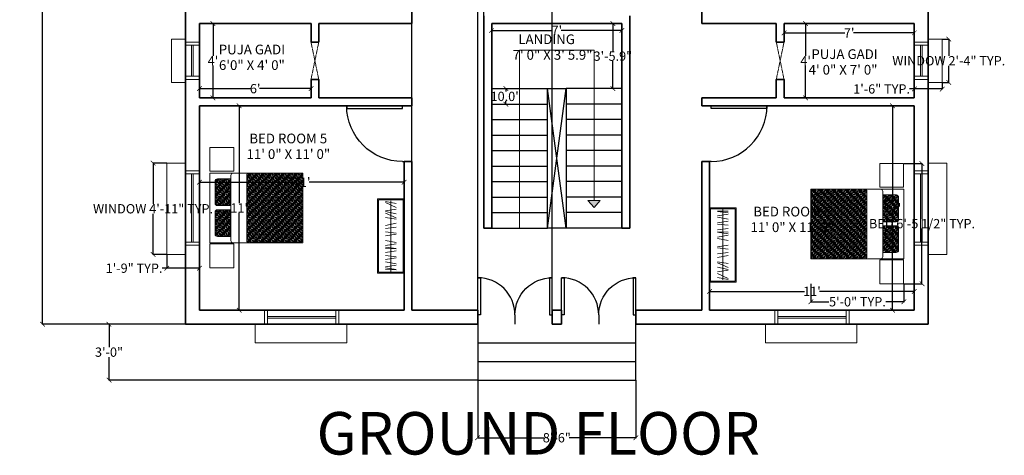
# Model space of a CAD drawing. Units: inches. Extents: x 844 to 2234, y 346 to 1084.
# Tile 1 of 93: x 844 to 1479, y 346 to 627. Entities that reach past the tile are written whole.
import ezdxf

# ---------------------------------------------------------------- set-up
doc = ezdxf.new("R2010")
doc.units = ezdxf.units.IN
doc.header["$MEASUREMENT"] = 0
doc.linetypes.add('DASHED', pattern=[0.75, 0.5, -0.25])
for name, color, linetype, lineweight in [('A-ANNO-DIMS', 2, 'Continuous', 18), ('A-ANNO-SYMB', 7, 'Continuous', 18), ('A-ANNO-TEXT', 7, 'Continuous', 35), ('A-AREA-IDEN', 7, 'Continuous', 18), ('A-FLOR-STRS', 7, 'Continuous', 25), ('A-WALL', 7, 'Continuous', 35), ('A-WALL-OVHD', 7, 'DASHED', 18), ('beds', 130, 'Continuous', 18), ('doors', 170, 'Continuous', 25), ('furniture', 8, 'Continuous', 18), ('windows', 1, 'Continuous', 18)]:
    doc.layers.add(name, color=color, linetype=linetype, lineweight=lineweight)
doc.styles.get("Standard").update_dxf_attribs({"font": 'arial.ttf'})
doc.dimstyles.get("Standard").update_dxf_attribs({"dimtxt": 6, "dimasz": 3, "dimexe": 0.18, "dimexo": 0.0625, "dimgap": 0.09, "dimtad": 0, "dimtih": 1, "dimtoh": 1, "dimdec": 1, "dimzin": 0, "dimdsep": 46, "dimlunit": 3, "dimtxsty": 'Standard', "dimblk": 'ARCHTICK', "dimcen": 0.09, "dimadec": 0, "dimazin": 0, "dimtfac": 1, "dimtdec": 1, "dimtofl": 0, "dimtmove": 0, "dimatfit": 3, "dimfxl": 1, "dimtolj": 1, "dimtzin": 0, "dimarcsym": 0})
pattern_1 = [(135, (-1377.70473, -125.71507), (-0.070710678, -0.070710678), []), (135, (-1377.68705, -125.69739), (-0.070710678, -0.070710678), []), (45, (-1377.70473, -125.71507), (-0.070710678, 0.070710678), [-0.025, 0.025]), (45, (-1377.72241, -125.69739), (-0.070710678, 0.070710678), [-0.025, 0.025]), (45, (-1377.74009, -125.67972), (-0.070710678, 0.070710678), [0.025, -0.025]), (45, (-1377.75776, -125.66204), (-0.070710678, 0.070710678), [0.025, -0.025]), (135, (-1377.66938, -125.67972), (-0.070710678, -0.070710678), [0.025, -0.025]), (135, (-1377.6517, -125.66204), (-0.070710678, -0.070710678), [0.025, -0.025])]

# ---------------------------------------------------------------- blocks, each defined once
blk = doc.blocks.new('*U2')
for p, q in [((0, 0), (0, -6)), ((36, 0), (36, -6))]:
    blk.add_line(p, q)
blk.add_lwpolyline([(0, 0), (0, 36), (1.75, 36), (1.75, 0)], close=True)
blk.add_arc((0, 0), 36, 0, 90)
blk = doc.blocks.new('*U4')
for p, q in [((0, 0), (0, -6)), ((24, 0), (24, -6))]:
    blk.add_line(p, q)
blk.add_lwpolyline([(0, 0), (0, 24), (1.75, 24), (1.75, 0)], close=True)
blk.add_arc((0, 0), 24, 0, 90)
blk = doc.blocks.new('MAT-P10')
h = blk.add_hatch()
h.set_pattern_fill('BOX', color=256, scale=0.1, angle=45, style=0)
h.set_pattern_definition(pattern_1)
h.paths.add_polyline_path([(-0.157, 1.46), (0.417, 1.46), (0.417, 1.751, 0.414214), (0.367, 1.801), (-0.107, 1.801, 0.414214), (-0.157, 1.751)])
h.paths.add_polyline_path([(0.505, 1.46), (1.079, 1.46), (1.079, 1.751, 0.414214), (1.029, 1.801), (0.555, 1.801, 0.414214), (0.505, 1.751)])
h = blk.add_hatch()
h.set_pattern_fill('BOX', color=256, scale=0.1, angle=45, style=0)
h.set_pattern_definition(pattern_1)
edge = h.paths.add_edge_path()
edge.add_line((1.205, -0.085), (1.205, 1.062))
edge.add_ellipse((1.161, 1.063), major_axis=(0, 0.0568), ratio=0.776379, start_angle=270, end_angle=360)
edge.add_line((1.161, 1.119), (-0.251, 1.12))
edge.add_ellipse((-0.251, 1.063), major_axis=(0, 0.0568), ratio=0.776379, start_angle=0, end_angle=88.1396)
edge.add_line((-0.295, 1.064), (-0.295, -0.085))
edge.add_line((-0.295, -0.085), (1.205, -0.085))
for p, q in [((-0.251, 1.46), (1.161, 1.46)), ((-0.251, 1.12), (1.161, 1.119)), ((1.102, 0.406), (1.102, 0.057)), ((1.058, 0), (0.775, 0))]:
    blk.add_line(p, q)
for points in [[(-0.83, 1.909), (-0.319, 1.909), (-0.319, 1.398), (-0.83, 1.398)], [(1.205, -0.085), (-0.295, -0.085), (-0.295, 1.915), (1.205, 1.915)], [(1.244, 1.909), (1.755, 1.909), (1.755, 1.398), (1.244, 1.398)]]:
    blk.add_lwpolyline(points, close=True)
for points in [[(0.417, 1.46), (0.417, 1.751, 0.414214), (0.367, 1.801), (-0.107, 1.801, 0.414214), (-0.157, 1.751), (-0.157, 1.46)], [(1.079, 1.46), (1.079, 1.751, 0.414214), (1.029, 1.801), (0.555, 1.801, 0.414214), (0.505, 1.751), (0.505, 1.46)], [(0.37, 1.624), (0.37, 1.571, -0.414214), (0.32, 1.521), (0.111, 1.521)], [(1.012, 1.644), (1.012, 1.571, -0.414214), (0.962, 1.521), (0.753, 1.521)]]:
    blk.add_lwpolyline(points, format="xyb")
at = {"extrusion": (0, 0, -1)}
for centre, start_param, end_param in [((-0.251, 1.404), 4.712389, 6.283185), ((1.161, 1.404), 0, 1.570796), ((-0.251, 1.063), 4.712389, 6.283185), ((1.161, 1.063), 0, 1.570796), ((1.058, 0.057), 1.570796, 3.141593), ((1.058, 0.057), 1.570796, 3.141593)]:
    blk.add_ellipse(centre, major_axis=(0, 0.0568), ratio=0.776379, start_param=start_param, end_param=end_param, dxfattribs=at)
blk = doc.blocks.new('A$C7A17768A')
for p, q in [((-2.8, 0), (0, 0)), ((-2.8, -1), (-2.8, 0)), ((0, -1), (0, 0)), ((-2.76, -0.04), (-0.04, -0.04)), ((-2.76, -0.96), (-2.76, -0.04)), ((-2.617, -0.3), (-2.694, -0.7)), ((-2.66, -0.7), (-2.466, -0.3)), ((-2.403, -0.3), (-2.342, -0.7)), ((-2.229, -0.296), (-2.317, -0.696)), ((-2.074, -0.3), (-2.25, -0.7)), ((-2.096, -0.7), (-2.033, -0.3)), ((-1.875, -0.3), (-1.796, -0.7)), ((-1.732, -0.3), (-1.675, -0.7)), ((-1.555, -0.7), (-1.507, -0.3)), ((-1.467, -0.3), (-1.403, -0.7)), ((-1.227, -0.7), (-1.151, -0.3)), ((-1.098, -0.3), (-1.034, -0.7)), ((-0.98, -0.7), (-0.921, -0.3)), ((-0.908, -0.3), (-0.919, -0.7)), ((-0.834, -0.3), (-0.777, -0.7)), ((-0.657, -0.7), (-0.61, -0.3)), ((-0.57, -0.3), (-0.505, -0.7)), ((-0.429, -0.7), (-0.353, -0.3)), ((-0.301, -0.3), (-0.237, -0.7)), ((-0.192, -0.7), (-0.133, -0.3)), ((-0.12, -0.3), (-0.131, -0.7)), ((-0.04, -0.96), (-0.04, -0.04)), ((-0.04, -0.5), (-2.716, -0.5)), ((-2.8, -1), (0, -1)), ((-2.76, -0.96), (-0.04, -0.96))]:
    blk.add_line(p, q)
blk = doc.blocks.new('_ArchTick')
at = {"color": 0, "linetype": 'ByBlock', "const_width": 0.15}
blk.add_lwpolyline([(-0.5, -0.5), (0.5, 0.5)], dxfattribs=at)
blk = doc.blocks.new('*D33')
at = {"layer": 'A-ANNO-DIMS', "color": 0, "lineweight": -2, "transparency": 16777216}
for p, q in [((1378.55, 624.31), (1350.37, 624.31)), ((1350.55, 624.31), (1350.55, 603.4)), ((1350.55, 576.31), (1350.55, 597.22)), ((1378.55, 576.31), (1350.37, 576.31))]:
    blk.add_line(p, q, dxfattribs=at)
at = {"layer": 'Defpoints', "color": 0, "transparency": 16777216}
for p in [(1378.62, 624.31), (1350.55, 576.31), (1378.62, 576.31)]:
    blk.add_point(p, dxfattribs=at)
at = {"layer": 'A-ANNO-DIMS', "color": 0, "lineweight": -2, "transparency": 16777216, "xscale": 3, "yscale": 3, "zscale": 3}
for p, rotation in [((1350.55, 624.31), 90), ((1350.55, 576.31), 270)]:
    blk.add_blockref('_ArchTick', p, dxfattribs=dict(at, rotation=rotation))
at = {"layer": 'A-ANNO-DIMS', "color": 0, "transparency": 16777216, "insert": (1350.55, 600.31), "char_height": 6, "attachment_point": 5}
blk.add_mtext("\\A1;4'", dxfattribs=at)
blk = doc.blocks.new('*D34')
at = {"layer": 'A-ANNO-DIMS', "color": 0, "lineweight": -2, "transparency": 16777216}
for p, q in [((1336.62, 618.37), (1336.62, 618.49)), ((1336.62, 618.31), (1375.79, 618.31)), ((1420.62, 618.31), (1381.44, 618.31)), ((1420.62, 618.37), (1420.62, 618.49))]:
    blk.add_line(p, q, dxfattribs=at)
at = {"layer": 'Defpoints', "color": 0, "transparency": 16777216}
for p in [(1336.62, 618.31), (1420.62, 618.31), (1420.62, 618.31)]:
    blk.add_point(p, dxfattribs=at)
at = {"layer": 'A-ANNO-DIMS', "color": 0, "lineweight": -2, "transparency": 16777216, "xscale": 3, "yscale": 3, "zscale": 3, "rotation": 180}
blk.add_blockref('_ArchTick', (1336.62, 618.31), dxfattribs=at)
at = {"layer": 'A-ANNO-DIMS', "color": 0, "lineweight": -2, "transparency": 16777216, "xscale": 3, "yscale": 3, "zscale": 3}
blk.add_blockref('_ArchTick', (1420.62, 618.31), dxfattribs=at)
at = {"layer": 'A-ANNO-DIMS', "color": 0, "transparency": 16777216, "insert": (1378.62, 618.31), "char_height": 6, "attachment_point": 5}
blk.add_mtext("\\A1;7'", dxfattribs=at)
blk = doc.blocks.new('*D35')
at = {"layer": 'A-ANNO-DIMS', "color": 0, "lineweight": -2, "transparency": 16777216}
for p, q in [((959.62, 580.55), (959.62, 582.49)), ((959.62, 582.31), (992.75, 582.31)), ((1031.62, 582.31), (998.48, 582.31)), ((1031.62, 580.55), (1031.62, 582.49))]:
    blk.add_line(p, q, dxfattribs=at)
at = {"layer": 'Defpoints', "color": 0, "transparency": 16777216}
for p in [(959.62, 580.49), (1031.62, 582.31), (1031.62, 580.49)]:
    blk.add_point(p, dxfattribs=at)
at = {"layer": 'A-ANNO-DIMS', "color": 0, "lineweight": -2, "transparency": 16777216, "xscale": 3, "yscale": 3, "zscale": 3, "rotation": 180}
blk.add_blockref('_ArchTick', (959.62, 582.31), dxfattribs=at)
at = {"layer": 'A-ANNO-DIMS', "color": 0, "lineweight": -2, "transparency": 16777216, "xscale": 3, "yscale": 3, "zscale": 3}
blk.add_blockref('_ArchTick', (1031.62, 582.31), dxfattribs=at)
at = {"layer": 'A-ANNO-DIMS', "color": 0, "transparency": 16777216, "insert": (995.62, 582.31), "char_height": 6, "attachment_point": 5}
blk.add_mtext("\\A1;6'", dxfattribs=at)
blk = doc.blocks.new('*D36')
at = {"layer": 'A-ANNO-DIMS', "color": 0, "lineweight": -2, "transparency": 16777216}
for p, q in [((968.62, 624.31), (968.25, 624.31)), ((968.43, 624.31), (968.43, 603.4)), ((968.43, 576.31), (968.43, 597.22)), ((968.62, 576.31), (968.25, 576.31))]:
    blk.add_line(p, q, dxfattribs=at)
at = {"layer": 'Defpoints', "color": 0, "transparency": 16777216}
for p in [(968.68, 624.31), (968.43, 576.31), (968.68, 576.31)]:
    blk.add_point(p, dxfattribs=at)
at = {"layer": 'A-ANNO-DIMS', "color": 0, "lineweight": -2, "transparency": 16777216, "xscale": 3, "yscale": 3, "zscale": 3}
for p, rotation in [((968.43, 624.31), 90), ((968.43, 576.31), 270)]:
    blk.add_blockref('_ArchTick', p, dxfattribs=dict(at, rotation=rotation))
at = {"layer": 'A-ANNO-DIMS', "color": 0, "transparency": 16777216, "insert": (968.43, 600.31), "char_height": 6, "attachment_point": 5}
blk.add_mtext("\\A1;4'", dxfattribs=at)
blk = doc.blocks.new('*D45')
at = {"layer": 'A-ANNO-DIMS', "color": 0, "lineweight": -2, "transparency": 16777216}
for p, q in [((965.15, 571.31), (985.47, 571.31)), ((985.29, 571.31), (985.29, 508.41)), ((985.29, 439.31), (985.29, 502.21)), ((965.15, 439.31), (985.47, 439.31))]:
    blk.add_line(p, q, dxfattribs=at)
at = {"layer": 'Defpoints', "color": 0, "transparency": 16777216}
for p in [(965.09, 571.31), (965.09, 439.31), (985.29, 439.31)]:
    blk.add_point(p, dxfattribs=at)
at = {"layer": 'A-ANNO-DIMS', "color": 0, "lineweight": -2, "transparency": 16777216, "xscale": 3, "yscale": 3, "zscale": 3}
for p, rotation in [((985.29, 571.31), 90), ((985.29, 439.31), 270)]:
    blk.add_blockref('_ArchTick', p, dxfattribs=dict(at, rotation=rotation))
at = {"layer": 'A-ANNO-DIMS', "color": 0, "transparency": 16777216, "insert": (985.29, 505.31), "char_height": 6, "attachment_point": 5}
blk.add_mtext("\\A1;11'", dxfattribs=at)
blk = doc.blocks.new('*D46')
at = {"layer": 'A-ANNO-DIMS', "color": 0, "lineweight": -2, "transparency": 16777216}
for p, q in [((959.62, 520.99), (959.62, 522.08)), ((959.62, 521.9), (1020.72, 521.9)), ((1091.62, 521.9), (1030.51, 521.9)), ((1091.62, 520.99), (1091.62, 522.08))]:
    blk.add_line(p, q, dxfattribs=at)
at = {"layer": 'Defpoints', "color": 0, "transparency": 16777216}
for p in [(959.62, 521.9), (959.62, 520.92), (1091.62, 520.92)]:
    blk.add_point(p, dxfattribs=at)
at = {"layer": 'A-ANNO-DIMS', "color": 0, "lineweight": -2, "transparency": 16777216, "xscale": 3, "yscale": 3, "zscale": 3, "rotation": 180}
blk.add_blockref('_ArchTick', (959.62, 521.9), dxfattribs=at)
at = {"layer": 'A-ANNO-DIMS', "color": 0, "lineweight": -2, "transparency": 16777216, "xscale": 3, "yscale": 3, "zscale": 3}
blk.add_blockref('_ArchTick', (1091.62, 521.9), dxfattribs=at)
at = {"layer": 'A-ANNO-DIMS', "color": 0, "transparency": 16777216, "insert": (1025.62, 521.9), "char_height": 6, "attachment_point": 5}
blk.add_mtext("\\A1;11'", dxfattribs=at)
blk = doc.blocks.new('*D47')
at = {"layer": 'A-ANNO-DIMS', "color": 0, "lineweight": -2, "transparency": 16777216}
for p, q in [((1288.62, 448.97), (1288.62, 451.69)), ((1288.62, 451.51), (1349.72, 451.51)), ((1420.62, 451.51), (1359.51, 451.51)), ((1420.62, 448.97), (1420.62, 451.69))]:
    blk.add_line(p, q, dxfattribs=at)
at = {"layer": 'Defpoints', "color": 0, "transparency": 16777216}
for p in [(1420.62, 451.51), (1288.62, 448.91), (1420.62, 448.91)]:
    blk.add_point(p, dxfattribs=at)
at = {"layer": 'A-ANNO-DIMS', "color": 0, "lineweight": -2, "transparency": 16777216, "xscale": 3, "yscale": 3, "zscale": 3, "rotation": 180}
blk.add_blockref('_ArchTick', (1288.62, 451.51), dxfattribs=at)
at = {"layer": 'A-ANNO-DIMS', "color": 0, "lineweight": -2, "transparency": 16777216, "xscale": 3, "yscale": 3, "zscale": 3}
blk.add_blockref('_ArchTick', (1420.62, 451.51), dxfattribs=at)
at = {"layer": 'A-ANNO-DIMS', "color": 0, "transparency": 16777216, "insert": (1354.62, 451.51), "char_height": 6, "attachment_point": 5}
blk.add_mtext("\\A1;11'", dxfattribs=at)
blk = doc.blocks.new('*D48')
at = {"layer": 'A-ANNO-DIMS', "color": 0, "lineweight": -2, "transparency": 16777216}
for p, q in [((1410.5, 571.31), (1406.35, 571.31)), ((1406.53, 571.31), (1406.53, 508.41)), ((1406.53, 439.31), (1406.53, 502.21)), ((1410.5, 439.31), (1406.35, 439.31))]:
    blk.add_line(p, q, dxfattribs=at)
at = {"layer": 'Defpoints', "color": 0, "transparency": 16777216}
for p in [(1410.56, 571.31), (1406.53, 439.31), (1410.56, 439.31)]:
    blk.add_point(p, dxfattribs=at)
at = {"layer": 'A-ANNO-DIMS', "color": 0, "lineweight": -2, "transparency": 16777216, "xscale": 3, "yscale": 3, "zscale": 3}
for p, rotation in [((1406.53, 571.31), 90), ((1406.53, 439.31), 270)]:
    blk.add_blockref('_ArchTick', p, dxfattribs=dict(at, rotation=rotation))
at = {"layer": 'A-ANNO-DIMS', "color": 0, "transparency": 16777216, "insert": (1406.53, 505.31), "char_height": 6, "attachment_point": 5}
blk.add_mtext("\\A1;11'", dxfattribs=at)
blk = doc.blocks.new('*D50')
at = {"layer": 'A-ANNO-DIMS', "color": 0, "lineweight": -2, "transparency": 16777216}
for p, q in [((1156.79, 582.31), (1157.46, 582.31)), ((1157.28, 582.31), (1157.28, 580.46)), ((1156.79, 572.31), (1157.46, 572.31)), ((1157.28, 572.31), (1157.28, 574.16))]:
    blk.add_line(p, q, dxfattribs=at)
at = {"layer": 'Defpoints', "color": 0, "transparency": 16777216}
for p in [(1156.72, 582.31), (1156.72, 572.31), (1157.28, 572.31)]:
    blk.add_point(p, dxfattribs=at)
at = {"layer": 'A-ANNO-DIMS', "color": 0, "lineweight": -2, "transparency": 16777216, "xscale": 3, "yscale": 3, "zscale": 3}
for p, rotation in [((1157.28, 582.31), 90), ((1157.28, 572.31), 270)]:
    blk.add_blockref('_ArchTick', p, dxfattribs=dict(at, rotation=rotation))
at = {"layer": 'A-ANNO-DIMS', "color": 0, "transparency": 16777216, "insert": (1157.28, 577.31), "char_height": 6, "attachment_point": 5}
blk.add_mtext('\\A1;10.0"', dxfattribs=at)
blk = doc.blocks.new('*D51')
at = {"layer": 'A-ANNO-DIMS', "color": 0, "lineweight": -2, "transparency": 16777216}
for p, q in [((1148.12, 619.91), (1148.12, 620.03)), ((1148.12, 619.85), (1187.29, 619.85)), ((1232.12, 619.85), (1192.94, 619.85)), ((1232.12, 619.91), (1232.12, 620.03))]:
    blk.add_line(p, q, dxfattribs=at)
at = {"layer": 'Defpoints', "color": 0, "transparency": 16777216}
for p in [(1148.12, 619.85), (1232.12, 619.85), (1232.12, 619.85)]:
    blk.add_point(p, dxfattribs=at)
at = {"layer": 'A-ANNO-DIMS', "color": 0, "lineweight": -2, "transparency": 16777216, "xscale": 3, "yscale": 3, "zscale": 3, "rotation": 180}
blk.add_blockref('_ArchTick', (1148.12, 619.85), dxfattribs=at)
at = {"layer": 'A-ANNO-DIMS', "color": 0, "lineweight": -2, "transparency": 16777216, "xscale": 3, "yscale": 3, "zscale": 3}
blk.add_blockref('_ArchTick', (1232.12, 619.85), dxfattribs=at)
at = {"layer": 'A-ANNO-DIMS', "color": 0, "transparency": 16777216, "insert": (1190.12, 619.85), "char_height": 6, "attachment_point": 5}
blk.add_mtext("\\A1;7'", dxfattribs=at)
blk = doc.blocks.new('*D52')
at = {"layer": 'A-ANNO-DIMS', "color": 0, "lineweight": -2, "transparency": 16777216}
for p, q in [((1226.23, 624.25), (1226.43, 624.25)), ((1226.25, 624.25), (1226.25, 606.44)), ((1226.25, 582.31), (1226.25, 600.13)), ((1226.23, 582.31), (1226.43, 582.31))]:
    blk.add_line(p, q, dxfattribs=at)
at = {"layer": 'Defpoints', "color": 0, "transparency": 16777216}
for p in [(1226.17, 624.25), (1226.17, 582.31), (1226.25, 582.31)]:
    blk.add_point(p, dxfattribs=at)
at = {"layer": 'A-ANNO-DIMS', "color": 0, "lineweight": -2, "transparency": 16777216, "xscale": 3, "yscale": 3, "zscale": 3}
for p, rotation in [((1226.25, 624.25), 90), ((1226.25, 582.31), 270)]:
    blk.add_blockref('_ArchTick', p, dxfattribs=dict(at, rotation=rotation))
at = {"layer": 'A-ANNO-DIMS', "color": 0, "transparency": 16777216, "insert": (1226.25, 603.28), "char_height": 6, "attachment_point": 5}
blk.add_mtext('\\A1;3\'-5.9"', dxfattribs=at)
blk = doc.blocks.new('*D56')
at = {"layer": 'A-ANNO-DIMS', "color": 0, "lineweight": -2, "transparency": 16777216}
for p, q in [((950.55, 1025.31), (858.33, 1025.31)), ((858.51, 1025.31), (858.51, 730.96)), ((858.51, 430.31), (858.51, 724.66)), ((950.55, 430.31), (858.33, 430.31))]:
    blk.add_line(p, q, dxfattribs=at)
at = {"layer": 'Defpoints', "color": 0, "transparency": 16777216}
for p in [(950.62, 1025.31), (858.51, 430.31), (950.62, 430.31)]:
    blk.add_point(p, dxfattribs=at)
at = {"layer": 'A-ANNO-DIMS', "color": 0, "lineweight": -2, "transparency": 16777216, "xscale": 3, "yscale": 3, "zscale": 3}
for p, rotation in [((858.51, 1025.31), 90), ((858.51, 430.31), 270)]:
    blk.add_blockref('_ArchTick', p, dxfattribs=dict(at, rotation=rotation))
at = {"layer": 'A-ANNO-DIMS', "color": 0, "transparency": 16777216, "insert": (858.51, 727.81), "char_height": 6, "attachment_point": 5}
blk.add_mtext('\\A1;49\'-7.0"', dxfattribs=at)
blk = doc.blocks.new('WIN-48IN')
for p, q in [((0, 9), (0, 21)), ((0, 21), (59, 21)), ((59, 9), (59, 21)), ((6, 9), (0, 9)), ((54, 9), (6, 9)), ((6, 9), (6, 0)), ((8, 9), (8, 0)), ((52, 0), (52, 9)), ((54, 0), (54, 9)), ((54, 9), (59, 9)), ((8, 5), (52, 5)), ((8, 4), (52, 4)), ((6, 0), (54, 0))]:
    blk.add_line(p, q)
blk = doc.blocks.new('WIN-24IN')
for p, q in [((9, 28), (0, 28)), ((0, 0), (0, 28)), ((9, 26), (9, 28)), ((18, 26), (9, 26)), ((9, 26), (9, 2)), ((18, 2), (18, 26)), ((18, 24), (9, 24)), ((13, 4), (13, 24)), ((14, 4), (14, 24)), ((9, 4), (18, 4)), ((9, 2), (18, 2)), ((9, 2), (9, 0)), ((9, 0), (0, 0))]:
    blk.add_line(p, q)
blk = doc.blocks.new('STAIR-RETURN-FLIGHTS')
for p, q in [((0, 90), (36, 90)), ((36, 0), (36, 90)), ((36, 90), (48, 90)), ((48, 0), (36, 90)), ((36, 0), (48, 90)), ((84, 90), (48, 90)), ((48, 90), (48, 0)), ((0, 80), (36, 80)), ((84, 80), (48, 80)), ((0, 70), (36, 70)), ((84, 70), (48, 70)), ((0, 60), (36, 60)), ((84, 60), (48, 60)), ((0, 50), (36, 50)), ((84, 50), (48, 50)), ((0, 40), (36, 40)), ((84, 40), (48, 40)), ((0, 30), (36, 30)), ((84, 30), (48, 30)), ((0, 20), (36, 20)), ((84, 20), (48, 20)), ((0, 10), (36, 10)), ((84, 10), (48, 10)), ((0, 0), (36, 0)), ((48, 0), (36, 0)), ((84, 0), (48, 0))]:
    blk.add_line(p, q)
blk = doc.blocks.new('STAIR-DIRECTION-RETURN')
h = blk.add_hatch(color=256)
h.dxf.hatch_style = 1
h.paths.add_polyline_path([(52, 17.85), (48, 17.85), (44, 17.85), (48, 13.33)])
for p, q in [((0, 0), (0, 114.78)), ((0, 114.78), (48, 114.78)), ((48, 114.78), (48, 17.85)), ((48, 17.85), (44, 17.85)), ((48, 13.33), (44, 17.85)), ((48, 17.85), (52, 17.85)), ((52, 17.85), (48, 13.33))]:
    blk.add_line(p, q)
blk = doc.blocks.new('*D103')
at = {"layer": 'A-ANNO-DIMS', "color": 0, "lineweight": -2, "transparency": 16777216}
for p, q in [((938.55, 534.31), (929.59, 534.31)), ((929.77, 534.31), (929.77, 508.01)), ((929.77, 475.31), (929.77, 501.62)), ((938.55, 475.31), (929.59, 475.31))]:
    blk.add_line(p, q, dxfattribs=at)
at = {"layer": 'Defpoints', "color": 0, "transparency": 16777216}
for p in [(929.77, 534.31), (938.62, 534.31), (938.62, 475.31)]:
    blk.add_point(p, dxfattribs=at)
at = {"layer": 'A-ANNO-DIMS', "color": 0, "lineweight": -2, "transparency": 16777216, "xscale": 3, "yscale": 3, "zscale": 3}
for p, rotation in [((929.77, 534.31), 90), ((929.77, 475.31), 270)]:
    blk.add_blockref('_ArchTick', p, dxfattribs=dict(at, rotation=rotation))
at = {"layer": 'A-ANNO-DIMS', "color": 0, "transparency": 16777216, "insert": (929.77, 504.81), "char_height": 6, "attachment_point": 5}
blk.add_mtext('\\A1;WINDOW 4\'-11" TYP.', dxfattribs=at)
blk = doc.blocks.new('*D104')
at = {"layer": 'A-ANNO-DIMS', "color": 0, "lineweight": -2, "transparency": 16777216}
for p, q in [((938.62, 475.25), (938.62, 466.28)), ((959.62, 475.25), (959.62, 466.28)), ((938.62, 466.46), (935.62, 466.46)), ((959.62, 466.46), (938.62, 466.46))]:
    blk.add_line(p, q, dxfattribs=at)
at = {"layer": 'Defpoints', "color": 0, "transparency": 16777216}
for p in [(938.62, 475.31), (959.62, 475.31), (938.62, 466.46)]:
    blk.add_point(p, dxfattribs=at)
at = {"layer": 'A-ANNO-DIMS', "color": 0, "lineweight": -2, "transparency": 16777216, "xscale": 3, "yscale": 3, "zscale": 3}
for p, rotation in [((938.62, 466.46), 179.9999999999992), ((959.62, 466.46), 359.9999999999992)]:
    blk.add_blockref('_ArchTick', p, dxfattribs=dict(at, rotation=rotation))
at = {"layer": 'A-ANNO-DIMS', "color": 0, "transparency": 16777216, "insert": (917.52, 466.46), "char_height": 6, "attachment_point": 5}
blk.add_mtext('\\A1;1\'-9" TYP.', dxfattribs=at)
blk = doc.blocks.new('*D105')
at = {"layer": 'A-ANNO-DIMS', "color": 0, "lineweight": -2, "transparency": 16777216}
for p, q in [((1414, 533.98), (1425.75, 533.98)), ((1425.57, 533.98), (1425.57, 498.4)), ((1425.57, 456.43), (1425.57, 492.02)), ((1414, 456.43), (1425.75, 456.43))]:
    blk.add_line(p, q, dxfattribs=at)
at = {"layer": 'Defpoints', "color": 0, "transparency": 16777216}
for p in [(1413.94, 533.98), (1425.57, 533.98), (1413.94, 456.43)]:
    blk.add_point(p, dxfattribs=at)
at = {"layer": 'A-ANNO-DIMS', "color": 0, "lineweight": -2, "transparency": 16777216, "xscale": 3, "yscale": 3, "zscale": 3}
for p, rotation in [((1425.57, 533.98), 90), ((1425.57, 456.43), 270)]:
    blk.add_blockref('_ArchTick', p, dxfattribs=dict(at, rotation=rotation))
at = {"layer": 'A-ANNO-DIMS', "color": 0, "transparency": 16777216, "insert": (1425.57, 495.21), "char_height": 6, "attachment_point": 5}
blk.add_mtext('\\A1;BED 6\'-5 1/2" TYP.', dxfattribs=at)
blk = doc.blocks.new('*D106')
at = {"layer": 'A-ANNO-DIMS', "color": 0, "lineweight": -2, "transparency": 16777216}
for p, q in [((1353.94, 456.37), (1353.94, 444.62)), ((1413.94, 456.37), (1413.94, 444.62)), ((1353.94, 444.8), (1365.56, 444.8)), ((1413.94, 444.8), (1402.31, 444.8))]:
    blk.add_line(p, q, dxfattribs=at)
at = {"layer": 'Defpoints', "color": 0, "transparency": 16777216}
for p in [(1353.94, 456.43), (1413.94, 456.43), (1413.94, 444.8)]:
    blk.add_point(p, dxfattribs=at)
at = {"layer": 'A-ANNO-DIMS', "color": 0, "lineweight": -2, "transparency": 16777216, "xscale": 3, "yscale": 3, "zscale": 3, "rotation": 180}
blk.add_blockref('_ArchTick', (1353.94, 444.8), dxfattribs=at)
at = {"layer": 'A-ANNO-DIMS', "color": 0, "lineweight": -2, "transparency": 16777216, "xscale": 3, "yscale": 3, "zscale": 3}
blk.add_blockref('_ArchTick', (1413.94, 444.8), dxfattribs=at)
at = {"layer": 'A-ANNO-DIMS', "color": 0, "transparency": 16777216, "insert": (1383.94, 444.8), "char_height": 6, "attachment_point": 5}
blk.add_mtext('\\A1;5\'-0" TYP.', dxfattribs=at)
blk = doc.blocks.new('*D109')
at = {"layer": 'A-ANNO-DIMS', "color": 0, "lineweight": -2, "transparency": 16777216}
for p, q in [((1438.68, 614.31), (1443, 614.31)), ((1442.82, 614.31), (1442.82, 603.51)), ((1442.82, 586.31), (1442.82, 597.12)), ((1438.68, 586.31), (1443, 586.31))]:
    blk.add_line(p, q, dxfattribs=at)
at = {"layer": 'Defpoints', "color": 0, "transparency": 16777216}
for p in [(1438.62, 614.31), (1438.62, 586.31), (1442.82, 586.31)]:
    blk.add_point(p, dxfattribs=at)
at = {"layer": 'A-ANNO-DIMS', "color": 0, "lineweight": -2, "transparency": 16777216, "xscale": 3, "yscale": 3, "zscale": 3}
for p, rotation in [((1442.82, 614.31), 90), ((1442.82, 586.31), 270)]:
    blk.add_blockref('_ArchTick', p, dxfattribs=dict(at, rotation=rotation))
at = {"layer": 'A-ANNO-DIMS', "color": 0, "transparency": 16777216, "insert": (1442.82, 600.31), "char_height": 6, "attachment_point": 5}
blk.add_mtext('\\A1;WINDOW 2\'-4" TYP.', dxfattribs=at)
blk = doc.blocks.new('*D110')
at = {"layer": 'A-ANNO-DIMS', "color": 0, "lineweight": -2, "transparency": 16777216}
for p, q in [((1420.62, 586.25), (1420.62, 581.93)), ((1438.62, 586.25), (1438.62, 581.93)), ((1420.62, 582.11), (1417.62, 582.11)), ((1438.62, 582.11), (1420.62, 582.11))]:
    blk.add_line(p, q, dxfattribs=at)
at = {"layer": 'Defpoints', "color": 0, "transparency": 16777216}
for p in [(1420.62, 586.31), (1438.62, 586.31), (1420.62, 582.11)]:
    blk.add_point(p, dxfattribs=at)
at = {"layer": 'A-ANNO-DIMS', "color": 0, "lineweight": -2, "transparency": 16777216, "xscale": 3, "yscale": 3, "zscale": 3, "rotation": 180}
blk.add_blockref('_ArchTick', (1420.62, 582.11), dxfattribs=at)
at = {"layer": 'A-ANNO-DIMS', "color": 0, "lineweight": -2, "transparency": 16777216, "xscale": 3, "yscale": 3, "zscale": 3}
blk.add_blockref('_ArchTick', (1438.62, 582.11), dxfattribs=at)
at = {"layer": 'A-ANNO-DIMS', "color": 0, "transparency": 16777216, "insert": (1399.52, 582.11), "char_height": 6, "attachment_point": 5}
blk.add_mtext('\\A1;1\'-6" TYP.', dxfattribs=at)
blk = doc.blocks.new('*D141')
at = {"layer": 'A-ANNO-DIMS', "color": 0, "lineweight": -2, "transparency": 16777216}
for p, q in [((1139.12, 394.25), (1139.12, 356.88)), ((1241.12, 394.25), (1241.12, 356.88)), ((1139.12, 357.06), (1182.05, 357.06)), ((1241.12, 357.06), (1198.18, 357.06))]:
    blk.add_line(p, q, dxfattribs=at)
at = {"layer": 'Defpoints', "color": 0, "transparency": 16777216}
for p in [(1139.12, 394.31), (1241.12, 394.31), (1241.12, 357.06)]:
    blk.add_point(p, dxfattribs=at)
at = {"layer": 'A-ANNO-DIMS', "color": 0, "lineweight": -2, "transparency": 16777216, "xscale": 3, "yscale": 3, "zscale": 3, "rotation": 180}
blk.add_blockref('_ArchTick', (1139.12, 357.06), dxfattribs=at)
at = {"layer": 'A-ANNO-DIMS', "color": 0, "lineweight": -2, "transparency": 16777216, "xscale": 3, "yscale": 3, "zscale": 3}
blk.add_blockref('_ArchTick', (1241.12, 357.06), dxfattribs=at)
at = {"layer": 'A-ANNO-DIMS', "color": 0, "transparency": 16777216, "insert": (1190.12, 357.06), "char_height": 6, "attachment_point": 5}
blk.add_mtext('\\A1;8\'-6"', dxfattribs=at)
blk = doc.blocks.new('*D142')
at = {"layer": 'A-ANNO-DIMS', "color": 0, "lineweight": -2, "transparency": 16777216}
for p, q in [((1139.05, 430.31), (901.19, 430.31)), ((901.37, 430.31), (901.37, 415.47)), ((901.37, 394.31), (901.37, 409.16)), ((1139.05, 394.31), (901.19, 394.31))]:
    blk.add_line(p, q, dxfattribs=at)
at = {"layer": 'Defpoints', "color": 0, "transparency": 16777216}
for p in [(901.37, 430.31), (1139.12, 430.31), (1139.12, 394.31)]:
    blk.add_point(p, dxfattribs=at)
at = {"layer": 'A-ANNO-DIMS', "color": 0, "lineweight": -2, "transparency": 16777216, "xscale": 3, "yscale": 3, "zscale": 3}
for p, rotation in [((901.37, 430.31), 90), ((901.37, 394.31), 270)]:
    blk.add_blockref('_ArchTick', p, dxfattribs=dict(at, rotation=rotation))
at = {"layer": 'A-ANNO-DIMS', "color": 0, "transparency": 16777216, "insert": (901.37, 412.31), "char_height": 6, "attachment_point": 5}
blk.add_mtext('\\A1;3\'-0"', dxfattribs=at)
blk = doc.blocks.new('*D143')
at = {"layer": 'A-ANNO-DIMS', "color": 0, "lineweight": -2, "transparency": 16777216}
for p, q in [((1139.12, 430.37), (1139.12, 1074.74)), ((1139.12, 1074.56), (1154.93, 1074.56)), ((1187.12, 1074.56), (1171.3, 1074.56)), ((1187.12, 430.37), (1187.12, 1074.74))]:
    blk.add_line(p, q, dxfattribs=at)
at = {"layer": 'Defpoints', "color": 0, "transparency": 16777216}
for p in [(1187.12, 1074.56), (1139.12, 430.31), (1187.12, 430.31)]:
    blk.add_point(p, dxfattribs=at)
at = {"layer": 'A-ANNO-DIMS', "color": 0, "lineweight": -2, "transparency": 16777216, "xscale": 3, "yscale": 3, "zscale": 3, "rotation": 180}
blk.add_blockref('_ArchTick', (1139.12, 1074.56), dxfattribs=at)
at = {"layer": 'A-ANNO-DIMS', "color": 0, "lineweight": -2, "transparency": 16777216, "xscale": 3, "yscale": 3, "zscale": 3}
blk.add_blockref('_ArchTick', (1187.12, 1074.56), dxfattribs=at)
at = {"layer": 'A-ANNO-DIMS', "color": 0, "transparency": 16777216, "insert": (1163.12, 1074.56), "char_height": 6, "attachment_point": 5}
blk.add_mtext('\\A1;4\'-0"', dxfattribs=at)
blk = doc.blocks.new('*D144')
at = {"layer": 'A-ANNO-DIMS', "color": 0, "lineweight": -2, "transparency": 16777216}
for p, q in [((1096.62, 439.37), (1096.62, 1074.74)), ((1096.62, 1074.56), (1102.48, 1074.56)), ((1143.12, 1074.56), (1137.25, 1074.56)), ((1143.12, 492.37), (1143.12, 1074.74))]:
    blk.add_line(p, q, dxfattribs=at)
at = {"layer": 'Defpoints', "color": 0, "transparency": 16777216}
for p in [(1143.12, 1074.56), (1143.12, 492.31), (1096.62, 439.31)]:
    blk.add_point(p, dxfattribs=at)
at = {"layer": 'A-ANNO-DIMS', "color": 0, "lineweight": -2, "transparency": 16777216, "xscale": 3, "yscale": 3, "zscale": 3, "rotation": 180}
blk.add_blockref('_ArchTick', (1096.62, 1074.56), dxfattribs=at)
at = {"layer": 'A-ANNO-DIMS', "color": 0, "lineweight": -2, "transparency": 16777216, "xscale": 3, "yscale": 3, "zscale": 3}
blk.add_blockref('_ArchTick', (1143.12, 1074.56), dxfattribs=at)
at = {"layer": 'A-ANNO-DIMS', "color": 0, "transparency": 16777216, "insert": (1119.87, 1074.56), "char_height": 6, "attachment_point": 5}
blk.add_mtext('\\A1;3\'-10 1/2"', dxfattribs=at)

msp = doc.modelspace()

# ---------------------------------------------------------------- linework, layer by layer
at = {"layer": 'A-FLOR-STRS'}
for p, q in [((1139.12, 430.31), (1139.12, 418.31)), ((1241.12, 418.31), (1241.12, 430.31)), ((1139.12, 418.31), (1241.12, 418.31)), ((1139.12, 418.31), (1139.12, 406.31)), ((1241.12, 406.31), (1241.12, 418.31)), ((1139.12, 406.31), (1241.12, 406.31)), ((1139.12, 406.31), (1139.12, 394.31)), ((1241.12, 394.31), (1241.12, 406.31)), ((1139.12, 394.31), (1241.12, 394.31))]:
    msp.add_line(p, q, dxfattribs=at)
at = {"layer": 'A-WALL'}
for p, q in [((950.62, 1025.31), (950.62, 430.31)), ((1429.62, 1025.31), (1429.62, 430.31)), ((1096.62, 761.31), (1096.62, 624.31)), ((1283.62, 761.31), (1283.62, 624.31)), ((1143.12, 629.31), (1143.12, 516.31)), ((1237.12, 629.31), (1237.12, 516.31)), ((959.62, 624.31), (1031.62, 624.31)), ((959.62, 624.31), (959.62, 576.31)), ((1031.62, 624.31), (1031.62, 612.31)), ((1036.62, 624.31), (1036.62, 612.31)), ((1036.62, 624.31), (1096.62, 624.31)), ((1148.12, 624.31), (1232.12, 624.31)), ((1148.12, 624.31), (1148.12, 516.31)), ((1232.12, 624.31), (1232.12, 516.31)), ((1331.62, 624.31), (1283.62, 624.31)), ((1331.62, 624.31), (1331.62, 612.31)), ((1420.62, 624.31), (1336.62, 624.31)), ((1336.62, 624.31), (1336.62, 612.31)), ((1420.62, 624.31), (1420.62, 576.31)), ((1036.62, 612.31), (1031.62, 612.31)), ((1331.62, 612.31), (1336.62, 612.31)), ((1036.62, 588.31), (1031.62, 588.31)), ((1031.62, 588.31), (1031.62, 576.31)), ((1036.62, 588.31), (1036.62, 576.31)), ((1331.62, 588.31), (1336.62, 588.31)), ((1331.62, 588.31), (1331.62, 576.31)), ((1336.62, 588.31), (1336.62, 576.31)), ((959.62, 576.31), (1031.62, 576.31)), ((1036.62, 576.31), (1096.62, 576.31)), ((1096.62, 571.31), (1096.62, 576.31)), ((1283.62, 576.31), (1283.62, 571.31)), ((1331.62, 576.31), (1283.62, 576.31)), ((1420.62, 576.31), (1336.62, 576.31)), ((959.62, 571.31), (1091.62, 571.31)), ((959.62, 571.31), (959.62, 439.31)), ((1091.62, 571.31), (1096.62, 571.31)), ((1288.62, 571.31), (1283.62, 571.31)), ((1420.62, 571.31), (1288.62, 571.31)), ((1420.62, 571.31), (1420.62, 439.31)), ((1091.62, 535.31), (1091.62, 439.31)), ((1091.62, 535.31), (1096.62, 535.31)), ((1096.62, 535.31), (1096.62, 439.31)), ((1288.62, 535.31), (1283.62, 535.31)), ((1283.62, 535.31), (1283.62, 439.31)), ((1288.62, 535.31), (1288.62, 439.31)), ((1143.12, 516.31), (1143.12, 492.31)), ((1148.12, 516.31), (1148.12, 492.31)), ((1232.12, 516.31), (1232.12, 492.31)), ((1237.12, 516.31), (1237.12, 492.31)), ((1143.12, 492.31), (1148.12, 492.31)), ((1237.12, 492.31), (1232.12, 492.31)), ((959.62, 439.31), (1091.62, 439.31)), ((1096.62, 439.31), (1139.12, 439.31)), ((1139.12, 439.31), (1139.12, 430.31)), ((1187.12, 439.31), (1187.12, 430.31)), ((1187.12, 439.31), (1193.12, 439.31)), ((1193.12, 439.31), (1193.12, 430.31)), ((1241.12, 439.31), (1241.12, 430.31)), ((1241.12, 439.31), (1283.62, 439.31)), ((1420.62, 439.31), (1288.62, 439.31)), ((950.62, 430.31), (1139.12, 430.31)), ((1187.12, 430.31), (1193.12, 430.31)), ((1241.12, 430.31), (1283.62, 430.31)), ((1429.62, 430.31), (1283.62, 430.31))]:
    msp.add_line(p, q, dxfattribs=at)
at = {"layer": 'A-WALL-OVHD'}
for p, q in [((1036.62, 588.31), (1031.62, 612.31)), ((1031.62, 588.31), (1036.62, 612.31)), ((1336.62, 588.31), (1331.62, 612.31)), ((1331.62, 588.31), (1336.62, 612.31))]:
    msp.add_line(p, q, dxfattribs=at)

# ---------------------------------------------------------------- block references
at = {"layer": 'A-ANNO-SYMB'}
msp.add_blockref('STAIR-DIRECTION-RETURN', (1166.12, 492.31), dxfattribs=at)
at = {"layer": 'A-FLOR-STRS'}
msp.add_blockref('STAIR-RETURN-FLIGHTS', (1148.12, 492.31), dxfattribs=at)
at = {"layer": 'beds', "yscale": 29.99962925113936, "zscale": 29.99962925113936}
for p, xscale, rotation in [((1023.75, 491.66), 29.99962925113936, 90), ((1356.48, 481.33), -29.99962925113936, 270)]:
    msp.add_blockref('MAT-P10', p, dxfattribs=dict(at, xscale=xscale, rotation=rotation))
at = {"layer": 'doors', "xscale": -1, "rotation": 90}
msp.add_blockref('*U2', (1090.62, 571.31), dxfattribs=at)
at = {"layer": 'doors', "rotation": 270}
msp.add_blockref('*U2', (1289.62, 571.31), dxfattribs=at)
at = {"layer": 'doors'}
for p in [(1139.12, 436.31), (1193.12, 436.31)]:
    msp.add_blockref('*U4', p, dxfattribs=at)
at = {"layer": 'doors', "xscale": -1}
for p in [(1187.12, 436.31), (1241.12, 436.31)]:
    msp.add_blockref('*U4', p, dxfattribs=at)
at = {"layer": 'furniture', "xscale": 17.14285714285603, "yscale": 17.14285714285603, "zscale": 17.14285714285603}
for p, rotation in [((1091.62, 463.31), 270), ((1288.62, 505.41), 90)]:
    msp.add_blockref('A$C7A17768A', p, dxfattribs=dict(at, rotation=rotation))
at = {"layer": 'windows'}
msp.add_blockref('WIN-24IN', (941.62, 586.31), dxfattribs=at)
for name, p, rotation in [('WIN-24IN', (1438.62, 614.31), 180), ('WIN-48IN', (959.62, 475.31), 89.9999999999992)]:
    msp.add_blockref(name, p, dxfattribs=dict(at, rotation=rotation))
at = {"layer": 'windows', "extrusion": (0, 0, -1), "zscale": -1}
for p, rotation in [((-1420.62, 475.31), 90.00000000000193), ((-995.62, 439.31), 180), ((-1324.62, 439.31), 180)]:
    msp.add_blockref('WIN-48IN', p, dxfattribs=dict(at, rotation=rotation))

# ---------------------------------------------------------------- texts
at = {"layer": 'A-ANNO-TEXT'}
msp.add_text('GROUND FLOOR', height=27.4468, dxfattribs=at).set_placement((1035.2, 346.21))
at = {"layer": 'A-AREA-IDEN'}
for s, height, p in [('LANDING', 6.269, (1165.29, 611.03)), ('PUJA GADI', 6.269, (972.13, 604.43)), ('7\' 0" X 3\' 5.9"', 6.2688, (1161.59, 600.96)), ('PUJA GADI', 6.269, (1354.25, 601.44)), ('  6\'0" X 4\' 0"', 6.2688, (968.43, 594.36)), (' 4\' 0" X 7\' 0"', 6.2688, (1350.55, 591.37)), ('BED ROOM 5', 6.269, (991.85, 547.02)), (' 11\' 0" X 11\' 0"', 6.2688, (988.15, 536.95)), ('BED ROOM 6', 6.269, (1316.8, 499.85)), (' 11\' 0" X 11\' 0"', 6.2688, (1313.11, 489.78))]:
    msp.add_text(s, height=height, dxfattribs=at).set_placement(p)

# ---------------------------------------------------------------- dimensions: what is measured, and where the dimension line sits
at = {"layer": 'A-ANNO-DIMS'}
for base, p1, p2, override, picture, middle in [((1143.12, 1074.56), (1096.62, 439.31), (1143.12, 492.31), {"dimdec": 1, "dimlfac": 1, "dimrnd": 0, "dimzin": 1, "dimdsep": 46, "dimlunit": 4, "dimfrac": 2}, '*D144', (1119.87, 1074.56)), ((1187.12, 1074.56), (1139.12, 430.31), (1187.12, 430.31), {"dimdec": 1, "dimlfac": 1, "dimrnd": 0, "dimzin": 1, "dimdsep": 46, "dimlunit": 4, "dimfrac": 2}, '*D143', (1163.12, 1074.56)), ((1232.12, 619.85), (1148.12, 619.85), (1232.12, 619.85), {"dimclrd": 0, "dimclre": 0, "dimclrt": 0}, '*D51', (1190.12, 619.85)), ((1420.62, 618.31), (1336.62, 618.31), (1420.62, 618.31), {"dimclrd": 0, "dimclre": 0, "dimclrt": 0}, '*D34', (1378.62, 618.31)), ((1031.62, 582.31), (959.62, 580.49), (1031.62, 580.49), {"dimclrd": 0, "dimclre": 0, "dimclrt": 0}, '*D35', (995.62, 582.31)), ((959.62, 521.9), (1091.62, 520.92), (959.62, 520.92), {"dimclrd": 0, "dimclre": 0, "dimclrt": 0}, '*D46', (1025.62, 521.9)), ((1420.62, 451.51), (1288.62, 448.91), (1420.62, 448.91), {"dimclrd": 0, "dimclre": 0, "dimclrt": 0}, '*D47', (1354.62, 451.51)), ((1241.12, 357.06), (1139.12, 394.31), (1241.12, 394.31), {"dimdec": 1, "dimlfac": 1, "dimrnd": 0, "dimzin": 1, "dimdsep": 46, "dimlunit": 4, "dimfrac": 2}, '*D141', (1190.12, 357.06))]:
    dim = msp.add_linear_dim(base=base, p1=p1, p2=p2, dimstyle='Standard', override=override, dxfattribs=at)
    dim.commit()
    dim.dimension.update_dxf_attribs({"geometry": picture, "text_midpoint": middle})
for base, p1, p2, override, picture, middle in [((858.51, 430.31), (950.62, 1025.31), (950.62, 430.31), {"dimclrd": 0, "dimclre": 0, "dimclrt": 0}, '*D56', (858.51, 727.81)), ((968.43, 576.31), (968.68, 624.31), (968.68, 576.31), {"dimclrd": 0, "dimclre": 0, "dimclrt": 0}, '*D36', (968.43, 600.31)), ((1226.25, 582.31), (1226.17, 624.25), (1226.17, 582.31), {"dimclrd": 0, "dimclre": 0, "dimclrt": 0}, '*D52', (1226.25, 603.28)), ((1350.55, 576.31), (1378.62, 624.31), (1378.62, 576.31), {"dimclrd": 0, "dimclre": 0, "dimclrt": 0}, '*D33', (1350.55, 600.31)), ((1157.28, 572.31), (1156.72, 582.31), (1156.72, 572.31), {"dimclrd": 0, "dimclre": 0, "dimclrt": 0}, '*D50', (1157.28, 577.31)), ((985.29, 439.31), (965.09, 571.31), (965.09, 439.31), {"dimclrd": 0, "dimclre": 0, "dimclrt": 0}, '*D45', (985.29, 505.31)), ((1406.53, 439.31), (1410.56, 571.31), (1410.56, 439.31), {"dimclrd": 0, "dimclre": 0, "dimclrt": 0}, '*D48', (1406.53, 505.31)), ((901.37, 430.31), (1139.12, 394.31), (1139.12, 430.31), {"dimdec": 1, "dimlfac": 1, "dimrnd": 0, "dimzin": 1, "dimdsep": 46, "dimlunit": 4, "dimfrac": 2}, '*D142', (901.37, 412.31))]:
    dim = msp.add_linear_dim(base=base, p1=p1, p2=p2, angle=90, dimstyle='Standard', override=override, dxfattribs=at)
    dim.commit()
    dim.dimension.update_dxf_attribs({"geometry": picture, "text_midpoint": middle})
for base, p1, p2, angle, text, picture, middle in [((1442.82, 586.31), (1438.62, 614.31), (1438.62, 586.31), 270, 'WINDOW <> TYP.', '*D109', (1442.82, 600.31)), ((1420.62, 582.11), (1438.62, 586.31), (1420.62, 586.31), 180, '<> TYP.', '*D110', (1399.52, 582.11)), ((929.77, 534.31), (938.62, 475.31), (938.62, 534.31), 90, 'WINDOW <> TYP.', '*D103', (929.77, 504.81)), ((1425.5687, 533.9839), (1413.9358, 456.4309), (1413.9358, 533.9839), 90, 'BED <> TYP.', '*D105', (1425.5687, 495.2074)), ((938.62, 466.46), (959.62, 475.31), (938.62, 475.31), 180, '<> TYP.', '*D104', (917.52, 466.46))]:
    dim = msp.add_linear_dim(base=base, p1=p1, p2=p2, angle=angle, text=text, dimstyle='Standard', override={"dimdec": 1, "dimlfac": 1, "dimrnd": 0, "dimzin": 1, "dimdsep": 46, "dimlunit": 4, "dimfrac": 2}, dxfattribs=at)
    dim.commit()
    dim.dimension.update_dxf_attribs({"geometry": picture, "text_midpoint": middle})
dim = msp.add_linear_dim(base=(1413.94, 444.8), p1=(1353.94, 456.43), p2=(1413.94, 456.43), text='<> TYP.', dimstyle='Standard', override={"dimdec": 1, "dimlfac": 1, "dimrnd": 0, "dimzin": 1, "dimdsep": 46, "dimlunit": 4, "dimfrac": 2}, dxfattribs=at)
dim.commit()
dim.dimension.update_dxf_attribs({"geometry": '*D106', "text_midpoint": (1383.94, 444.8)})

doc.saveas('drawing.dxf')
